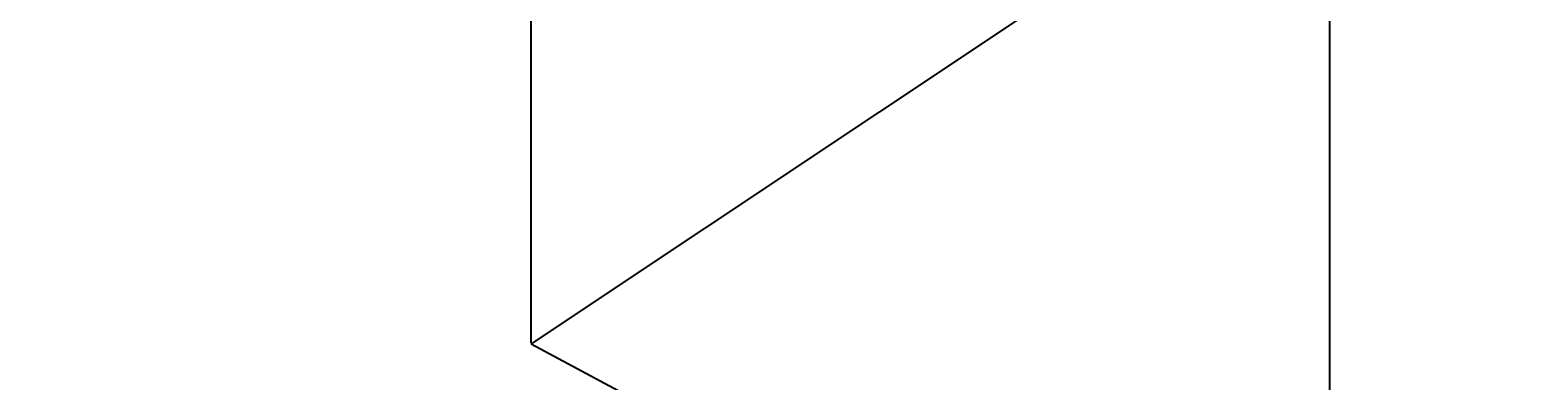
# Model space of a CAD drawing. Units: inches. Extents: x 35362 to 73946, y 43607 to 67532.
# Tile 119 of 134: x 50905 to 51049, y 49095 to 49128. Entities that reach past the tile are written whole.
import ezdxf

# ---------------------------------------------------------------- set-up
doc = ezdxf.new("R2010")
doc.units = ezdxf.units.IN
doc.header["$MEASUREMENT"] = 0
doc.layers.add('A-ANNO-DIMS', color=2, linetype='Continuous', lineweight=18)
doc.layers.add('E-SYMB', color=1, linetype='Continuous', lineweight=25)
doc.styles.get("Standard").update_dxf_attribs({"font": 'arial.ttf'})
doc.dimstyles.get("Standard").update_dxf_attribs({"dimtxt": 0.18, "dimasz": 0.18, "dimexe": 0.18, "dimexo": 0.0625, "dimgap": 0.09, "dimtad": 0, "dimtih": 1, "dimtoh": 1, "dimdec": 4, "dimzin": 0, "dimdsep": 46, "dimtxsty": 'Standard', "dimcen": 0.09, "dimadec": 0, "dimazin": 0, "dimtfac": 1, "dimtdec": 4, "dimtofl": 0, "dimtmove": 0, "dimatfit": 3, "dimfxl": 1, "dimtolj": 1, "dimtzin": 0, "dimarcsym": 0})

# ---------------------------------------------------------------- blocks, each defined once
blk = doc.blocks.new('*D11')
at = {"layer": 'A-ANNO-DIMS', "color": 0, "lineweight": -2, "transparency": 16777216}
for p, q in [((47978.66, 56028.77), (47978.66, 43606.68)), ((53109.76, 56028.77), (53109.76, 43606.68)), ((47978.84, 43606.86), (50543.87, 43606.86)), ((53109.58, 43606.86), (50544.55, 43606.86))]:
    blk.add_line(p, q, dxfattribs=at)
at = {"layer": 'A-ANNO-DIMS', "color": 0, "transparency": 16777216}
for points in [[(47978.84, 43606.89), (47978.84, 43606.83), (47978.66, 43606.86)], [(53109.58, 43606.89), (53109.58, 43606.83), (53109.76, 43606.86)]]:
    blk.add_solid(points, dxfattribs=at)
at = {"layer": 'Defpoints', "color": 0, "transparency": 16777216}
for p in [(47978.66, 56028.84), (53109.76, 56028.84), (53109.76, 43606.86)]:
    blk.add_point(p, dxfattribs=at)
at = {"layer": 'A-ANNO-DIMS', "color": 0, "transparency": 16777216, "insert": (50544.21, 43606.86), "char_height": 0.18, "attachment_point": 5}
blk.add_mtext('\\A1;5131', dxfattribs=at)
blk = doc.blocks.new('*D13')
at = {"layer": 'A-ANNO-DIMS', "color": 0, "lineweight": -2, "transparency": 16777216}
for p, q in [((48373.49, 51694.02), (48373.49, 43606.68)), ((51029.04, 51694.02), (51029.04, 43606.68)), ((48373.67, 43606.86), (49700.8, 43606.86)), ((51028.86, 43606.86), (49701.73, 43606.86))]:
    blk.add_line(p, q, dxfattribs=at)
at = {"layer": 'A-ANNO-DIMS', "color": 0, "transparency": 16777216}
for points in [[(48373.67, 43606.89), (48373.67, 43606.83), (48373.49, 43606.86)], [(51028.86, 43606.89), (51028.86, 43606.83), (51029.04, 43606.86)]]:
    blk.add_solid(points, dxfattribs=at)
at = {"layer": 'Defpoints', "color": 0, "transparency": 16777216}
for p in [(48373.49, 51694.09), (51029.04, 51694.09), (51029.04, 43606.86)]:
    blk.add_point(p, dxfattribs=at)
at = {"layer": 'A-ANNO-DIMS', "color": 0, "transparency": 16777216, "insert": (49701.27, 43606.86), "char_height": 0.18, "attachment_point": 5}
blk.add_mtext('\\A1;2655.6', dxfattribs=at)
blk = doc.blocks.new('*D17')
at = {"layer": 'A-ANNO-DIMS', "color": 0, "lineweight": -2, "transparency": 16777216}
for p, q in [((49923.31, 61293.22), (49923.31, 43606.68)), ((51913.93, 61293.22), (51913.93, 43606.68)), ((49923.49, 43606.86), (50918.16, 43606.86)), ((51913.75, 43606.86), (50919.07, 43606.86))]:
    blk.add_line(p, q, dxfattribs=at)
at = {"layer": 'A-ANNO-DIMS', "color": 0, "transparency": 16777216}
for points in [[(49923.49, 43606.89), (49923.49, 43606.83), (49923.31, 43606.86)], [(51913.75, 43606.89), (51913.75, 43606.83), (51913.93, 43606.86)]]:
    blk.add_solid(points, dxfattribs=at)
at = {"layer": 'Defpoints', "color": 0, "transparency": 16777216}
for p in [(49923.31, 61293.29), (51913.93, 61293.29), (51913.93, 43606.86)]:
    blk.add_point(p, dxfattribs=at)
at = {"layer": 'A-ANNO-DIMS', "color": 0, "transparency": 16777216, "insert": (50918.62, 43606.86), "char_height": 0.18, "attachment_point": 5}
blk.add_mtext('\\A1;1990.6', dxfattribs=at)
blk = doc.blocks.new('*D67')
at = {"layer": 'A-ANNO-DIMS', "color": 0, "lineweight": -2, "transparency": 16777216}
for p, q in [((56873.54, 53351.53), (35361.77, 53351.53)), ((35361.95, 53351.35), (35361.95, 49400.89)), ((35361.95, 45450.07), (35361.95, 49400.53)), ((53793.58, 45449.89), (35361.77, 45449.89))]:
    blk.add_line(p, q, dxfattribs=at)
at = {"layer": 'A-ANNO-DIMS', "color": 0, "transparency": 16777216}
for points in [[(35361.92, 53351.35), (35361.98, 53351.35), (35361.95, 53351.53)], [(35361.92, 45450.07), (35361.98, 45450.07), (35361.95, 45449.89)]]:
    blk.add_solid(points, dxfattribs=at)
at = {"layer": 'Defpoints', "color": 0, "transparency": 16777216}
for p in [(35361.95, 53351.53), (56873.6, 53351.53), (53793.64, 45449.89)]:
    blk.add_point(p, dxfattribs=at)
at = {"layer": 'A-ANNO-DIMS', "color": 0, "transparency": 16777216, "insert": (35361.95, 49400.71), "char_height": 0.18, "attachment_point": 5}
blk.add_mtext('\\A1;7901.6', dxfattribs=at)
blk = doc.blocks.new('*D84')
at = {"layer": 'A-ANNO-DIMS', "color": 0, "lineweight": -2, "transparency": 16777216}
for p, q in [((55540.23, 49259.94), (35361.77, 49259.94)), ((35361.95, 49259.76), (35361.95, 49115.14)), ((35361.95, 48970.16), (35361.95, 49114.78)), ((55540.23, 48969.98), (35361.77, 48969.98))]:
    blk.add_line(p, q, dxfattribs=at)
at = {"layer": 'A-ANNO-DIMS', "color": 0, "transparency": 16777216}
for points in [[(35361.92, 49259.76), (35361.98, 49259.76), (35361.95, 49259.94)], [(35361.92, 48970.16), (35361.98, 48970.16), (35361.95, 48969.98)]]:
    blk.add_solid(points, dxfattribs=at)
at = {"layer": 'Defpoints', "color": 0, "transparency": 16777216}
for p in [(35361.95, 49259.94), (55540.3, 49259.94), (55540.3, 48969.98)]:
    blk.add_point(p, dxfattribs=at)
at = {"layer": 'A-ANNO-DIMS', "color": 0, "transparency": 16777216, "insert": (35361.95, 49114.96), "char_height": 0.18, "attachment_point": 5}
blk.add_mtext('\\A1;289.96', dxfattribs=at)
blk = doc.blocks.new('*D85')
at = {"layer": 'A-ANNO-DIMS', "color": 0, "lineweight": -2, "transparency": 16777216}
for p, q in [((50952.66, 49098.43), (50952.66, 67531.69)), ((51285.59, 49320.14), (51285.59, 67531.69)), ((50952.84, 67531.51), (51118.73, 67531.51)), ((51285.41, 67531.51), (51119.52, 67531.51))]:
    blk.add_line(p, q, dxfattribs=at)
at = {"layer": 'A-ANNO-DIMS', "color": 0, "transparency": 16777216}
for points in [[(50952.84, 67531.54), (50952.84, 67531.48), (50952.66, 67531.51)], [(51285.41, 67531.54), (51285.41, 67531.48), (51285.59, 67531.51)]]:
    blk.add_solid(points, dxfattribs=at)
at = {"layer": 'Defpoints', "color": 0, "transparency": 16777216}
for p in [(51285.59, 67531.51), (51285.59, 49320.08), (50952.66, 49098.37)]:
    blk.add_point(p, dxfattribs=at)
at = {"layer": 'A-ANNO-DIMS', "color": 0, "transparency": 16777216, "insert": (51119.13, 67531.51), "char_height": 0.18, "attachment_point": 5}
blk.add_mtext('\\A1;332.9', dxfattribs=at)
blk = doc.blocks.new('*D86')
at = {"layer": 'A-ANNO-DIMS', "color": 0, "lineweight": -2, "transparency": 16777216}
for p, q in [((51285.53, 49320.08), (35361.77, 49320.08)), ((35361.95, 49319.9), (35361.95, 49120.26)), ((35361.95, 48920.26), (35361.95, 49119.9)), ((51285.53, 48920.08), (35361.77, 48920.08))]:
    blk.add_line(p, q, dxfattribs=at)
at = {"layer": 'A-ANNO-DIMS', "color": 0, "transparency": 16777216}
for points in [[(35361.92, 49319.9), (35361.98, 49319.9), (35361.95, 49320.08)], [(35361.92, 48920.26), (35361.98, 48920.26), (35361.95, 48920.08)]]:
    blk.add_solid(points, dxfattribs=at)
at = {"layer": 'Defpoints', "color": 0, "transparency": 16777216}
for p in [(35361.95, 49320.08), (51285.59, 49320.08), (51285.59, 48920.08)]:
    blk.add_point(p, dxfattribs=at)
at = {"layer": 'A-ANNO-DIMS', "color": 0, "transparency": 16777216, "insert": (35361.95, 49120.08), "char_height": 0.18, "attachment_point": 5}
blk.add_mtext('\\A1;400.0', dxfattribs=at)
blk = doc.blocks.new('*D107')
at = {"layer": 'A-ANNO-DIMS', "color": 0, "lineweight": -2, "transparency": 16777216}
for p, q in [((50139.56, 59850.01), (50139.56, 43606.68)), ((51320.81, 59850.01), (51320.81, 43606.68)), ((50139.74, 43606.86), (50729.73, 43606.86)), ((51320.63, 43606.86), (50730.64, 43606.86))]:
    blk.add_line(p, q, dxfattribs=at)
at = {"layer": 'A-ANNO-DIMS', "color": 0, "transparency": 16777216}
for points in [[(50139.74, 43606.89), (50139.74, 43606.83), (50139.56, 43606.86)], [(51320.63, 43606.89), (51320.63, 43606.83), (51320.81, 43606.86)]]:
    blk.add_solid(points, dxfattribs=at)
at = {"layer": 'Defpoints', "color": 0, "transparency": 16777216}
for p in [(50139.56, 59850.08), (51320.81, 59850.08), (51320.81, 43606.86)]:
    blk.add_point(p, dxfattribs=at)
at = {"layer": 'A-ANNO-DIMS', "color": 0, "transparency": 16777216, "insert": (50730.19, 43606.86), "char_height": 0.18, "attachment_point": 5}
blk.add_mtext('\\A1;1181.3', dxfattribs=at)

msp = doc.modelspace()

# ---------------------------------------------------------------- linework, layer by layer
at = {"layer": 'E-SYMB'}
for p, q in [((51285.595, 49320.079), (50952.662, 49098.368)), ((50952.662, 49098.368), (51285.595, 48920.079))]:
    msp.add_line(p, q, dxfattribs=at)

# ---------------------------------------------------------------- dimensions: what is measured, and where the dimension line sits
at = {"layer": 'A-ANNO-DIMS'}
for base, p1, p2, override, picture, middle in [((51285.595, 67531.512), (50952.662, 49098.368), (51285.595, 49320.079), {"dimdec": 1, "dimlfac": 1, "dimrnd": 0, "dimzin": 0, "dimdsep": 46, "dimlunit": 2}, '*D85', (51119.128, 67531.512)), ((51913.931, 43606.859), (49923.307, 61293.286), (51913.931, 61293.286), {"dimdec": 1, "dimlfac": 1, "dimrnd": 0, "dimzin": 0, "dimdsep": 46, "dimlunit": 2}, '*D17', (50918.619, 43606.859)), ((51320.8133, 43606.859), (50139.5627, 59850.0769), (51320.8133, 59850.0769), {"dimdec": 1, "dimlfac": 1, "dimrnd": 0, "dimzin": 0, "dimdsep": 46, "dimlunit": 2}, '*D107', (50730.188, 43606.859)), ((53109.76, 43606.859), (47978.665, 56028.836), (53109.76, 56028.836), {"dimdec": 0, "dimlfac": 1, "dimrnd": 0, "dimzin": 0, "dimdsep": 46, "dimlunit": 2}, '*D11', (50544.212, 43606.859)), ((51029.043, 43606.859), (48373.492, 51694.087), (51029.043, 51694.087), {"dimdec": 1, "dimlfac": 1, "dimrnd": 0, "dimzin": 0, "dimdsep": 46, "dimlunit": 2}, '*D13', (49701.267, 43606.859))]:
    dim = msp.add_linear_dim(base=base, p1=p1, p2=p2, dimstyle='Standard', override=override, dxfattribs=at)
    dim.commit()
    dim.dimension.update_dxf_attribs({"geometry": picture, "text_midpoint": middle})
for base, p1, p2, override, picture, middle in [((35361.949, 53351.529), (53793.638, 45449.894), (56873.602, 53351.529), {"dimdec": 1, "dimlfac": 1, "dimrnd": 0, "dimzin": 0, "dimdsep": 46, "dimlunit": 2}, '*D67', (35361.949, 49400.712)), ((35361.949, 49320.079), (51285.595, 48920.079), (51285.595, 49320.079), {"dimdec": 1, "dimlfac": 1, "dimrnd": 0, "dimzin": 0, "dimdsep": 46, "dimlunit": 2}, '*D86', (35361.949, 49120.079)), ((35361.9491, 49259.9353), (55540.2972, 48969.9796), (55540.2972, 49259.9353), {"dimdec": 2, "dimlfac": 1, "dimrnd": 0, "dimzin": 0, "dimdsep": 46, "dimlunit": 2}, '*D84', (35361.9491, 49114.9575))]:
    dim = msp.add_linear_dim(base=base, p1=p1, p2=p2, angle=90, dimstyle='Standard', override=override, dxfattribs=at)
    dim.commit()
    dim.dimension.update_dxf_attribs({"geometry": picture, "text_midpoint": middle})

doc.saveas('drawing.dxf')
